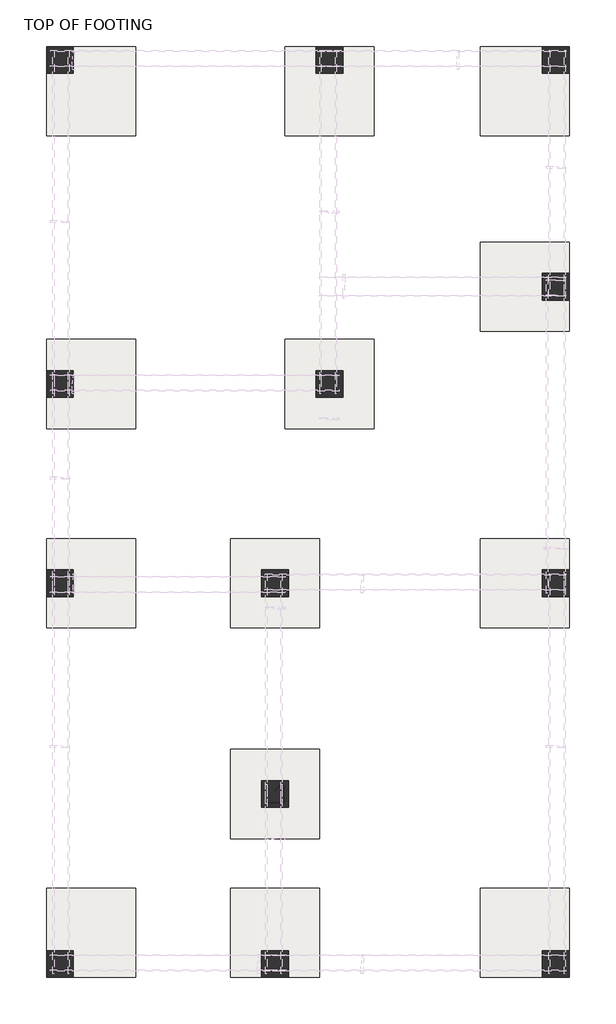
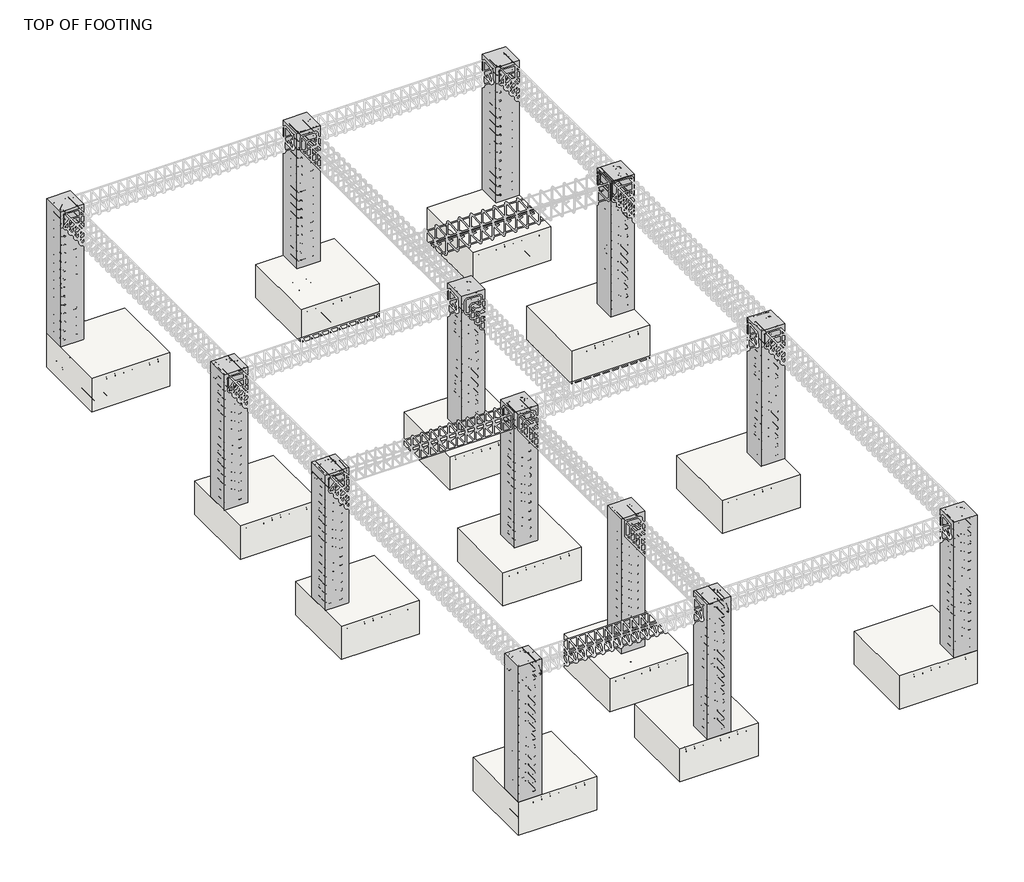
# One storey, part 1 of 10: 13 columns, 13 slabs.
"""IFC4 building model written with IfcOpenShell, lengths in millimetres."""

from ifc_helpers import new_model, si_unit, frame, origin, place, context, project, spatial, polyline, outline, extrude, transform, mapped, element, save
from components import m_footing_rectangular_1000mm_x_1000mm_x_450mm_4c97ae35

model = new_model("IFC4")

# Units and contexts
model_context = context("Model", 3, world=origin())
ifc_project = project(units=[si_unit("LENGTHUNIT", "METRE", prefix="MILLI")], contexts=[model_context])

# Site, building, storey
site = spatial("IfcSite", under=ifc_project)
building = spatial("IfcBuilding", under=site)
storey = spatial("IfcBuildingStorey", under=building, Name="TOP OF FOOTING", Elevation=-1828.8)

# Columns
placement = place(None, origin())
element("IfcColumn", 1, ObjectType="M_Concrete-Rectangular-Column : 300MM X 300MM", at=placement, inside=storey, context=model_context, shape_type="SweptSolid", body=[
    extrude(outline(polyline([(-10391.0457678, 18346.8267485), (-10391.0457678, 18046.8267485), (-10691.0457678, 18046.8267485), (-10691.0457678, 18346.8267485), (-10391.0457678, 18346.8267485)])), frame((0.0, 0.0, -1828.8), z_axis=(0.0, 0.0, 1.0), x_axis=(1.0, 0.0, 0.0)), (0.0, 0.0, 1.0), 1828.8),
])
element("IfcColumn", 2, ObjectType="M_Concrete-Rectangular-Column : 300MM X 300MM", at=placement, inside=storey, context=model_context, shape_type="SweptSolid", body=[
    extrude(outline(polyline([(-7366.0457678, 18346.8267485), (-7366.0457678, 18046.8267485), (-7666.0457678, 18046.8267485), (-7666.0457678, 18346.8267485), (-7366.0457678, 18346.8267485)])), frame((0.0, 0.0, -1828.8), z_axis=(0.0, 0.0, 1.0), x_axis=(1.0, 0.0, 0.0)), (0.0, 0.0, 1.0), 1828.8),
])
element("IfcColumn", 3, ObjectType="M_Concrete-Rectangular-Column : 300MM X 300MM", at=placement, inside=storey, context=model_context, shape_type="SweptSolid", body=[
    extrude(outline(polyline([(-4823.6457678, 18346.8267485), (-4823.6457678, 18046.8267485), (-5123.6457678, 18046.8267485), (-5123.6457678, 18346.8267485), (-4823.6457678, 18346.8267485)])), frame((0.0, 0.0, -1828.8), z_axis=(0.0, 0.0, 1.0), x_axis=(1.0, 0.0, 0.0)), (0.0, 0.0, 1.0), 1828.8),
])
element("IfcColumn", 4, ObjectType="M_Concrete-Rectangular-Column : 300MM X 300MM", at=placement, inside=storey, context=model_context, shape_type="SweptSolid", body=[
    extrude(outline(polyline([(-10391.0457678, 14712.2267485), (-10391.0457678, 14412.2267485), (-10691.0457678, 14412.2267485), (-10691.0457678, 14712.2267485), (-10391.0457678, 14712.2267485)])), frame((0.0, 0.0, -1828.8), z_axis=(0.0, 0.0, 1.0), x_axis=(1.0, 0.0, 0.0)), (0.0, 0.0, 1.0), 1828.8),
])
element("IfcColumn", 5, ObjectType="M_Concrete-Rectangular-Column : 300MM X 300MM", at=placement, inside=storey, context=model_context, shape_type="SweptSolid", body=[
    extrude(outline(polyline([(-7366.0457678, 14712.2267485), (-7366.0457678, 14412.2267485), (-7666.0457678, 14412.2267485), (-7666.0457678, 14712.2267485), (-7366.0457678, 14712.2267485)])), frame((0.0, 0.0, -1828.8), z_axis=(0.0, 0.0, 1.0), x_axis=(1.0, 0.0, 0.0)), (0.0, 0.0, 1.0), 1828.8),
])
element("IfcColumn", 6, ObjectType="M_Concrete-Rectangular-Column : 300MM X 300MM", at=placement, inside=storey, context=model_context, shape_type="SweptSolid", body=[
    extrude(outline(polyline([(-4823.6457678, 15804.4267485), (-4823.6457678, 15504.4267485), (-5123.6457678, 15504.4267485), (-5123.6457678, 15804.4267485), (-4823.6457678, 15804.4267485)])), frame((0.0, 0.0, -1828.8), z_axis=(0.0, 0.0, 1.0), x_axis=(1.0, 0.0, 0.0)), (0.0, 0.0, 1.0), 1828.8),
])
element("IfcColumn", 7, ObjectType="M_Concrete-Rectangular-Column : 300MM X 300MM", at=placement, inside=storey, context=model_context, shape_type="SweptSolid", body=[
    extrude(outline(polyline([(-7975.6457678, 8207.4267485), (-7975.6457678, 7907.4267485), (-8275.6457678, 7907.4267485), (-8275.6457678, 8207.4267485), (-7975.6457678, 8207.4267485)])), frame((0.0, 0.0, -1828.8), z_axis=(0.0, 0.0, 1.0), x_axis=(1.0, 0.0, 0.0)), (0.0, 0.0, 1.0), 1828.8),
])
element("IfcColumn", 8, ObjectType="M_Concrete-Rectangular-Column : 300MM X 300MM", at=placement, inside=storey, context=model_context, shape_type="SweptSolid", body=[
    extrude(outline(polyline([(-10391.0457678, 8207.4267485), (-10391.0457678, 7907.4267485), (-10691.0457678, 7907.4267485), (-10691.0457678, 8207.4267485), (-10391.0457678, 8207.4267485)])), frame((0.0, 0.0, -1828.8), z_axis=(0.0, 0.0, 1.0), x_axis=(1.0, 0.0, 0.0)), (0.0, 0.0, 1.0), 1828.8),
])
element("IfcColumn", 9, ObjectType="M_Concrete-Rectangular-Column : 300MM X 300MM", at=placement, inside=storey, context=model_context, shape_type="SweptSolid", body=[
    extrude(outline(polyline([(-10391.0457678, 12477.0267485), (-10391.0457678, 12177.0267485), (-10691.0457678, 12177.0267485), (-10691.0457678, 12477.0267485), (-10391.0457678, 12477.0267485)])), frame((0.0, 0.0, -1828.8), z_axis=(0.0, 0.0, 1.0), x_axis=(1.0, 0.0, 0.0)), (0.0, 0.0, 1.0), 1828.8),
])
element("IfcColumn", 10, ObjectType="M_Concrete-Rectangular-Column : 300MM X 300MM", at=placement, inside=storey, context=model_context, shape_type="SweptSolid", body=[
    extrude(outline(polyline([(-7975.6457678, 12477.0267485), (-7975.6457678, 12177.0267485), (-8275.6457678, 12177.0267485), (-8275.6457678, 12477.0267485), (-7975.6457678, 12477.0267485)])), frame((0.0, 0.0, -1828.8), z_axis=(0.0, 0.0, 1.0), x_axis=(1.0, 0.0, 0.0)), (0.0, 0.0, 1.0), 1828.8),
])
element("IfcColumn", 11, ObjectType="M_Concrete-Rectangular-Column : 300MM X 300MM", at=placement, inside=storey, context=model_context, shape_type="SweptSolid", body=[
    extrude(outline(polyline([(-4823.6457678, 12477.0267485), (-4823.6457678, 12177.0267485), (-5123.6457678, 12177.0267485), (-5123.6457678, 12477.0267485), (-4823.6457678, 12477.0267485)])), frame((0.0, 0.0, -1828.8), z_axis=(0.0, 0.0, 1.0), x_axis=(1.0, 0.0, 0.0)), (0.0, 0.0, 1.0), 1828.8),
])
element("IfcColumn", 12, ObjectType="M_Concrete-Rectangular-Column : 300MM X 300MM", at=placement, inside=storey, context=model_context, shape_type="SweptSolid", body=[
    extrude(outline(polyline([(-4823.6457678, 8207.4267485), (-4823.6457678, 7907.4267485), (-5123.6457678, 7907.4267485), (-5123.6457678, 8207.4267485), (-4823.6457678, 8207.4267485)])), frame((0.0, 0.0, -1828.8), z_axis=(0.0, 0.0, 1.0), x_axis=(1.0, 0.0, 0.0)), (0.0, 0.0, 1.0), 1828.8),
])
element("IfcColumn", 13, ObjectType="M_Concrete-Rectangular-Column : 300MM X 300MM", at=placement, inside=storey, context=model_context, shape_type="SweptSolid", body=[
    extrude(outline(polyline([(-7975.6457678, 10114.8267485), (-7975.6457678, 9814.8267485), (-8275.6457678, 9814.8267485), (-8275.6457678, 10114.8267485), (-7975.6457678, 10114.8267485)])), frame((0.0, 0.0, -1828.8), z_axis=(0.0, 0.0, 1.0), x_axis=(1.0, 0.0, 0.0)), (0.0, 0.0, 1.0), 1828.8),
])

# Slabs
m_footing_rectangular_1000mm_x_1000mm_x_450mm_shape = m_footing_rectangular_1000mm_x_1000mm_x_450mm_4c97ae35(model_context)
element("IfcSlab", 14, ObjectType="M_Footing-Rectangular : 1000MM X 1000MM X 450MM", at=placement, inside=storey, context=model_context, shape_type="MappedRepresentation", body=[
    mapped(m_footing_rectangular_1000mm_x_1000mm_x_450mm_shape, transform((-10191.0457678, 17846.8267485, -1828.8), x_axis=(1.0, 0.0, 0.0), y_axis=(0.0, 1.0, 0.0), z_axis=(0.0, 0.0, 1.0))),
])
element("IfcSlab", 15, ObjectType="M_Footing-Rectangular : 1000MM X 1000MM X 450MM", at=placement, inside=storey, context=model_context, shape_type="MappedRepresentation", body=[
    mapped(m_footing_rectangular_1000mm_x_1000mm_x_450mm_shape, transform((-7516.0457678, 17846.8267485, -1828.8), x_axis=(1.0, 0.0, 0.0), y_axis=(0.0, 1.0, 0.0), z_axis=(0.0, 0.0, 1.0))),
])
element("IfcSlab", 16, ObjectType="M_Footing-Rectangular : 1000MM X 1000MM X 450MM", at=placement, inside=storey, context=model_context, shape_type="MappedRepresentation", body=[
    mapped(m_footing_rectangular_1000mm_x_1000mm_x_450mm_shape, transform((-5323.6457678, 17846.8267485, -1828.8), x_axis=(1.0, 0.0, 0.0), y_axis=(0.0, 1.0, 0.0), z_axis=(0.0, 0.0, 1.0))),
])
element("IfcSlab", 17, ObjectType="M_Footing-Rectangular : 1000MM X 1000MM X 450MM", at=placement, inside=storey, context=model_context, shape_type="MappedRepresentation", body=[
    mapped(m_footing_rectangular_1000mm_x_1000mm_x_450mm_shape, transform((-5323.6457678, 15654.4267485, -1828.8), x_axis=(1.0, 0.0, 0.0), y_axis=(0.0, 1.0, 0.0), z_axis=(0.0, 0.0, 1.0))),
])
element("IfcSlab", 18, ObjectType="M_Footing-Rectangular : 1000MM X 1000MM X 450MM", at=placement, inside=storey, context=model_context, shape_type="MappedRepresentation", body=[
    mapped(m_footing_rectangular_1000mm_x_1000mm_x_450mm_shape, transform((-7516.0457678, 14562.2267485, -1828.8), x_axis=(1.0, 0.0, 0.0), y_axis=(0.0, 1.0, 0.0), z_axis=(0.0, 0.0, 1.0))),
])
element("IfcSlab", 19, ObjectType="M_Footing-Rectangular : 1000MM X 1000MM X 450MM", at=placement, inside=storey, context=model_context, shape_type="MappedRepresentation", body=[
    mapped(m_footing_rectangular_1000mm_x_1000mm_x_450mm_shape, transform((-10191.0457678, 14562.2267485, -1828.8), x_axis=(1.0, 0.0, 0.0), y_axis=(0.0, 1.0, 0.0), z_axis=(0.0, 0.0, 1.0))),
])
element("IfcSlab", 20, ObjectType="M_Footing-Rectangular : 1000MM X 1000MM X 450MM", at=placement, inside=storey, context=model_context, shape_type="MappedRepresentation", body=[
    mapped(m_footing_rectangular_1000mm_x_1000mm_x_450mm_shape, transform((-10191.0457678, 12327.0267485, -1828.8), x_axis=(1.0, 0.0, 0.0), y_axis=(0.0, 1.0, 0.0), z_axis=(0.0, 0.0, 1.0))),
])
element("IfcSlab", 21, ObjectType="M_Footing-Rectangular : 1000MM X 1000MM X 450MM", at=placement, inside=storey, context=model_context, shape_type="MappedRepresentation", body=[
    mapped(m_footing_rectangular_1000mm_x_1000mm_x_450mm_shape, transform((-10191.0457678, 8407.4267485, -1828.8), x_axis=(1.0, 0.0, 0.0), y_axis=(0.0, 1.0, 0.0), z_axis=(0.0, 0.0, 1.0))),
])
element("IfcSlab", 22, ObjectType="M_Footing-Rectangular : 1000MM X 1000MM X 450MM", at=placement, inside=storey, context=model_context, shape_type="MappedRepresentation", body=[
    mapped(m_footing_rectangular_1000mm_x_1000mm_x_450mm_shape, transform((-8125.6457678, 8407.4267485, -1828.8), x_axis=(1.0, 0.0, 0.0), y_axis=(0.0, 1.0, 0.0), z_axis=(0.0, 0.0, 1.0))),
])
element("IfcSlab", 23, ObjectType="M_Footing-Rectangular : 1000MM X 1000MM X 450MM", at=placement, inside=storey, context=model_context, shape_type="MappedRepresentation", body=[
    mapped(m_footing_rectangular_1000mm_x_1000mm_x_450mm_shape, transform((-5323.6457678, 8407.4267485, -1828.8), x_axis=(1.0, 0.0, 0.0), y_axis=(0.0, 1.0, 0.0), z_axis=(0.0, 0.0, 1.0))),
])
element("IfcSlab", 24, ObjectType="M_Footing-Rectangular : 1000MM X 1000MM X 450MM", at=placement, inside=storey, context=model_context, shape_type="MappedRepresentation", body=[
    mapped(m_footing_rectangular_1000mm_x_1000mm_x_450mm_shape, transform((-8125.6457678, 9964.8267485, -1828.8), x_axis=(1.0, 0.0, 0.0), y_axis=(0.0, 1.0, 0.0), z_axis=(0.0, 0.0, 1.0))),
])
element("IfcSlab", 25, ObjectType="M_Footing-Rectangular : 1000MM X 1000MM X 450MM", at=placement, inside=storey, context=model_context, shape_type="MappedRepresentation", body=[
    mapped(m_footing_rectangular_1000mm_x_1000mm_x_450mm_shape, transform((-8125.6457678, 12327.0267485, -1828.8), x_axis=(1.0, 0.0, 0.0), y_axis=(0.0, 1.0, 0.0), z_axis=(0.0, 0.0, 1.0))),
])
element("IfcSlab", 26, ObjectType="M_Footing-Rectangular : 1000MM X 1000MM X 450MM", at=placement, inside=storey, context=model_context, shape_type="MappedRepresentation", body=[
    mapped(m_footing_rectangular_1000mm_x_1000mm_x_450mm_shape, transform((-5323.6457678, 12327.0267485, -1828.8), x_axis=(1.0, 0.0, 0.0), y_axis=(0.0, 1.0, 0.0), z_axis=(0.0, 0.0, 1.0))),
])

save(model, "model.ifc")

# Revit data of these elements
# Grids (mm)
#   "D": line (-8125.646, 11185.604) -> (-8125.646, 6045.054)
#   "A": line (-10691.046, 19297.11) -> (-10691.046, 6421.116)
#   "B": line (-7516.046, 19297.11) -> (-7516.046, 13625.066)
#   "C": line (-4823.646, 19297.11) -> (-4823.646, 6421.116)
#   "1": line (-2439.679, 18346.827) -> (-11729.639, 18346.827)
#   "3": line (-2439.679, 14562.227) -> (-11729.639, 14562.227)
#   "4": line (-2439.679, 12327.027) -> (-11729.639, 12327.027)
#   "6": line (-2439.679, 7907.427) -> (-11729.639, 7907.427)
#   "2": line (-2439.679, 15654.427) -> (-6569.194, 15654.427)
#   "5": line (-2439.679, 9964.827) -> (-8972.917, 9964.827)
# Type "M_Concrete-Rectangular-Column : 300MM X 300MM"
#   b = 300 mm
#   h = 300 mm
#   Structural Material [instance default] = Concrete, Cast-in-Place gray
# Type "M_Footing-Rectangular : 1000MM X 1000MM X 450MM"
#   Width = 1000 mm
#   Length = 1000 mm
#   Foundation Thickness = 450 mm
#   Structural Material [instance default] = Concrete, Cast-in-Place gray
#   Assembly Code = ""
# Elements 1, 2, 3, 4, 5, 6, 7, 8, 9, 10, 11, 12, 13 (IfcColumn, "M_Concrete-Rectangular-Column : 300MM X 300MM")
#   Structural Material = Concrete, Cast-in-Place gray
#   Phase Created = New Construction
#   Materials on its faces: "Concrete, Cast-in-Place gray"
# Elements 14, 15, 16, 17, 18, 19, 20, 21, 22, 23, 24, 25, 26 (IfcSlab, "M_Footing-Rectangular : 1000MM X 1000MM X 450MM")
#   Structural Material = Concrete, Cast-in-Place gray
#   Phase Created = New Construction
#   Materials on its faces: "Concrete, Cast-in-Place gray"
# Materials
#   "Concrete, Cast-in-Place gray": class "Concrete", colour RGB 192 192 192, transparency 0, Description = "Cast-in-place concrete", Cost = 0
